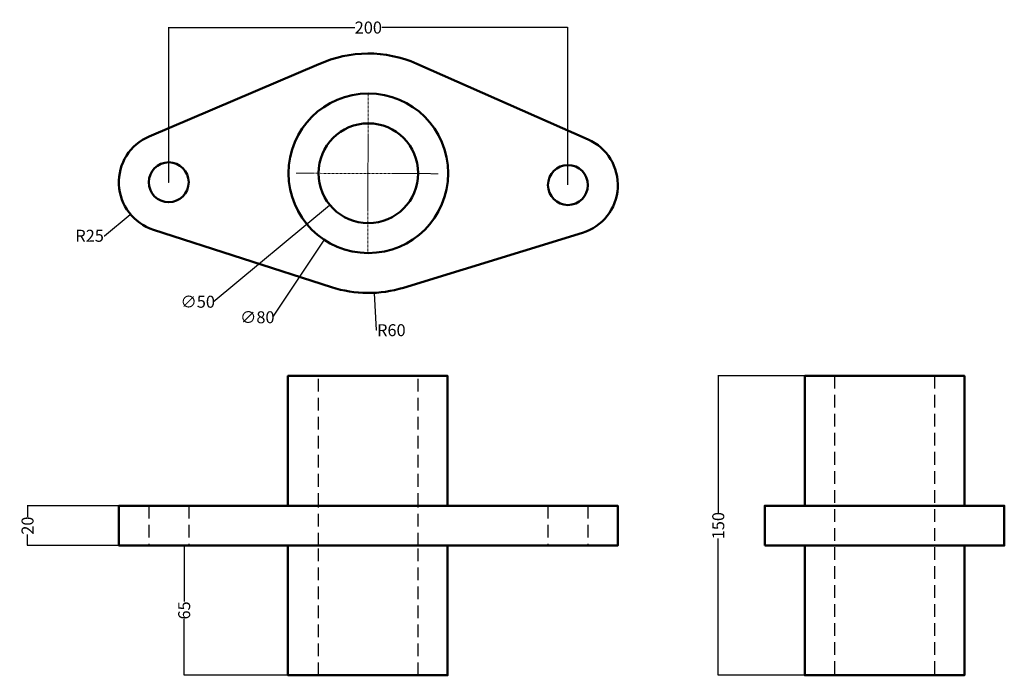
# Model space of a CAD drawing. Units: millimetres. Extents: x 110 to 603, y -63 to 265.
import ezdxf

# ---------------------------------------------------------------- set-up
doc = ezdxf.new("R2010")
doc.units = ezdxf.units.MM
doc.header["$MEASUREMENT"] = 0
doc.linetypes.add('CENTER', pattern=[2, 1.25, -0.25, 0.25, -0.25])
doc.linetypes.add('HIDDEN', pattern=[9.525, 6.35, -3.175])
for name, color, linetype, lineweight in [('M-CNTR', 4, 'CENTER', 18), ('M-DIMS', 2, 'Continuous', 25), ('M-HIDN', 1, 'HIDDEN', 25), ('M-OUTL', 7, 'Continuous', 50)]:
    doc.layers.add(name, color=color, linetype=linetype, lineweight=lineweight)
doc.styles.get("Standard").update_dxf_attribs({"font": 'arial.ttf'})
doc.dimstyles.get("Standard").update_dxf_attribs({"dimtxt": 6, "dimasz": 0.18, "dimexe": 0.18, "dimexo": 0.0625, "dimgap": 0.09, "dimtad": 0, "dimtoh": 1, "dimdec": 0, "dimzin": 0, "dimdsep": 46, "dimtxsty": 'Standard', "dimcen": 0.09, "dimadec": 0, "dimazin": 0, "dimtfac": 1, "dimtdec": 0, "dimtofl": 0, "dimtmove": 0, "dimatfit": 3, "dimfxl": 1, "dimtolj": 1, "dimtzin": 0, "dimarcsym": 0})

# ---------------------------------------------------------------- blocks, each defined once
blk = doc.blocks.new('*D1')
at = {"layer": 'Defpoints', "color": 0, "transparency": 16777216}
for p in [(384.64, 261.41), (184.64, 183.88), (384.64, 182.49)]:
    blk.add_point(p, dxfattribs=at)
at = {"layer": 'M-DIMS', "color": 0, "lineweight": -2, "transparency": 16777216}
for p, q in [((184.64, 183.94), (184.64, 261.59)), ((384.64, 182.55), (384.64, 261.59)), ((184.82, 261.41), (277.88, 261.41)), ((384.46, 261.41), (291.4, 261.41))]:
    blk.add_line(p, q, dxfattribs=at)
at = {"layer": 'M-DIMS', "color": 0, "transparency": 16777216}
for points in [[(184.82, 261.44), (184.82, 261.38), (184.64, 261.41)], [(384.46, 261.44), (384.46, 261.38), (384.64, 261.41)]]:
    blk.add_solid(points, dxfattribs=at)
at = {"layer": 'M-DIMS', "color": 0, "transparency": 16777216, "insert": (284.64, 261.41), "char_height": 6, "attachment_point": 5}
blk.add_mtext('\\A1;200', dxfattribs=at)
blk = doc.blocks.new('*D2')
at = {"layer": 'Defpoints', "color": 0, "transparency": 16777216}
for p in [(184.64, 183.88), (165.43, 167.88)]:
    blk.add_point(p, dxfattribs=at)
at = {"layer": 'M-DIMS', "color": 0, "lineweight": -2, "transparency": 16777216}
for p, q in [((184.55, 183.88), (184.73, 183.88)), ((184.64, 183.79), (184.64, 183.97)), ((152.45, 157.07), (165.29, 167.77)), ((152.27, 157.07), (152.45, 157.07))]:
    blk.add_line(p, q, dxfattribs=at)
at = {"layer": 'M-DIMS', "color": 0, "transparency": 16777216}
blk.add_solid([(165.27, 167.79), (165.31, 167.74), (165.43, 167.88)], dxfattribs=at)
at = {"layer": 'M-DIMS', "color": 0, "transparency": 16777216, "insert": (144.99, 157.07), "char_height": 6, "attachment_point": 5}
blk.add_mtext('\\A1;R25', dxfattribs=at)
blk = doc.blocks.new('*D3')
at = {"layer": 'Defpoints', "color": 0, "transparency": 16777216}
for p in [(284.64, 188.4), (287.76, 128.48)]:
    blk.add_point(p, dxfattribs=at)
at = {"layer": 'M-DIMS', "color": 0, "lineweight": -2, "transparency": 16777216}
for p, q in [((284.55, 188.4), (284.73, 188.4)), ((284.64, 188.31), (284.64, 188.49)), ((288.74, 109.76), (287.77, 128.3)), ((288.92, 109.76), (288.74, 109.76))]:
    blk.add_line(p, q, dxfattribs=at)
at = {"layer": 'M-DIMS', "color": 0, "transparency": 16777216}
blk.add_solid([(287.8, 128.3), (287.74, 128.3), (287.76, 128.48)], dxfattribs=at)
at = {"layer": 'M-DIMS', "color": 0, "transparency": 16777216, "insert": (296.17, 109.76), "char_height": 6, "attachment_point": 5}
blk.add_mtext('\\A1;R60', dxfattribs=at)
blk = doc.blocks.new('*D4')
at = {"layer": 'Defpoints', "color": 0, "transparency": 16777216}
for p in [(303.89, 204.35), (265.39, 172.44)]:
    blk.add_point(p, dxfattribs=at)
at = {"layer": 'M-DIMS', "color": 0, "lineweight": -2, "transparency": 16777216}
for p, q in [((284.55, 188.4), (284.73, 188.4)), ((284.64, 188.31), (284.64, 188.49)), ((206.97, 124.02), (265.25, 172.33)), ((206.79, 124.02), (206.97, 124.02))]:
    blk.add_line(p, q, dxfattribs=at)
at = {"layer": 'M-DIMS', "color": 0, "transparency": 16777216}
blk.add_solid([(265.23, 172.35), (265.27, 172.31), (265.39, 172.44)], dxfattribs=at)
at = {"layer": 'M-DIMS', "color": 0, "transparency": 16777216, "insert": (199.15, 124.02), "char_height": 6, "attachment_point": 5}
blk.add_mtext('\\A1;∅50', dxfattribs=at)
blk = doc.blocks.new('*D5')
at = {"layer": 'Defpoints', "color": 0, "transparency": 16777216}
for p in [(306.73, 221.74), (262.54, 155.06)]:
    blk.add_point(p, dxfattribs=at)
at = {"layer": 'M-DIMS', "color": 0, "lineweight": -2, "transparency": 16777216}
for p, q in [((284.55, 188.4), (284.73, 188.4)), ((284.64, 188.31), (284.64, 188.49)), ((236.82, 116.24), (262.44, 154.91)), ((236.64, 116.24), (236.82, 116.24))]:
    blk.add_line(p, q, dxfattribs=at)
at = {"layer": 'M-DIMS', "color": 0, "transparency": 16777216}
blk.add_solid([(262.42, 154.92), (262.47, 154.89), (262.54, 155.06)], dxfattribs=at)
at = {"layer": 'M-DIMS', "color": 0, "transparency": 16777216, "insert": (229, 116.24), "char_height": 6, "attachment_point": 5}
blk.add_mtext('\\A1;∅80', dxfattribs=at)
blk = doc.blocks.new('*D6')
at = {"layer": 'Defpoints', "color": 0, "transparency": 16777216}
for p in [(113.9, 21.82), (167.53, 21.82), (167.53, 1.82)]:
    blk.add_point(p, dxfattribs=at)
at = {"layer": 'M-DIMS', "color": 0, "lineweight": -2, "transparency": 16777216}
for p, q in [((167.46, 21.82), (113.72, 21.82)), ((113.9, 21.64), (113.9, 16.24)), ((113.9, 2), (113.9, 7.39)), ((167.46, 1.82), (113.72, 1.82))]:
    blk.add_line(p, q, dxfattribs=at)
at = {"layer": 'M-DIMS', "color": 0, "transparency": 16777216}
for points in [[(113.87, 21.64), (113.93, 21.64), (113.9, 21.82)], [(113.87, 2), (113.93, 2), (113.9, 1.82)]]:
    blk.add_solid(points, dxfattribs=at)
at = {"layer": 'M-DIMS', "color": 0, "transparency": 16777216, "insert": (113.9, 11.82), "char_height": 6, "attachment_point": 5, "rotation": 90}
blk.add_mtext('\\A1;20', dxfattribs=at)
blk = doc.blocks.new('*D7')
at = {"layer": 'Defpoints', "color": 0, "transparency": 16777216}
for p in [(244.32, 1.82), (192.38, -63.18), (244.32, -63.18)]:
    blk.add_point(p, dxfattribs=at)
at = {"layer": 'M-DIMS', "color": 0, "lineweight": -2, "transparency": 16777216}
for p, q in [((244.26, 1.82), (192.2, 1.82)), ((192.38, 1.64), (192.38, -26.26)), ((192.38, -63), (192.38, -35.11)), ((244.26, -63.18), (192.2, -63.18))]:
    blk.add_line(p, q, dxfattribs=at)
at = {"layer": 'M-DIMS', "color": 0, "transparency": 16777216}
for points in [[(192.35, 1.64), (192.41, 1.64), (192.38, 1.82)], [(192.35, -63), (192.41, -63), (192.38, -63.18)]]:
    blk.add_solid(points, dxfattribs=at)
at = {"layer": 'M-DIMS', "color": 0, "transparency": 16777216, "insert": (192.38, -30.68), "char_height": 6, "attachment_point": 5, "rotation": 90}
blk.add_mtext('\\A1;65', dxfattribs=at)
blk = doc.blocks.new('*D8')
at = {"layer": 'Defpoints', "color": 0, "transparency": 16777216}
for p in [(543.27, 86.82), (459.96, -63.18), (543.27, -63.18)]:
    blk.add_point(p, dxfattribs=at)
at = {"layer": 'M-DIMS', "color": 0, "lineweight": -2, "transparency": 16777216}
for p, q in [((543.21, 86.82), (459.78, 86.82)), ((459.96, 86.64), (459.96, 18.24)), ((459.96, -63), (459.96, 5.39)), ((543.21, -63.18), (459.78, -63.18))]:
    blk.add_line(p, q, dxfattribs=at)
at = {"layer": 'M-DIMS', "color": 0, "transparency": 16777216}
for points in [[(459.93, 86.64), (459.99, 86.64), (459.96, 86.82)], [(459.93, -63), (459.99, -63), (459.96, -63.18)]]:
    blk.add_solid(points, dxfattribs=at)
at = {"layer": 'M-DIMS', "color": 0, "transparency": 16777216, "insert": (459.96, 11.82), "char_height": 6, "attachment_point": 5, "rotation": 90}
blk.add_mtext('\\A1;150', dxfattribs=at)

msp = doc.modelspace()

# ---------------------------------------------------------------- linework, layer by layer
at = {"layer": 'M-CNTR'}
for p, q in [((284.58, 228.4), (284.33, 148.4)), ((248.5, 188.4), (319.7, 188.18))]:
    msp.add_line(p, q, dxfattribs=at)
at = {"layer": 'M-HIDN'}
for p, q in [((518.27, 86.82), (518.27, -63.18)), ((568.27, 86.82), (568.27, -63.18)), ((174.64, 21.82), (174.64, 1.82)), ((194.64, 21.82), (194.64, 1.82)), ((374.64, 21.82), (374.64, 1.82)), ((394.64, 21.82), (394.64, 1.82))]:
    msp.add_line(p, q, dxfattribs=at)
for points in [[(259.64, -63.18), (259.64, 1.82), (259.64, 21.82), (259.64, 86.82)], [(309.64, -63.18), (309.64, 1.82), (309.64, 21.82), (309.64, 86.82)]]:
    msp.add_lwpolyline(points, dxfattribs=at)
at = {"layer": 'M-OUTL'}
msp.add_lwpolyline([(174.85, 206.89, 0.69424), (176.96, 160.09), (266.22, 131.3, 0.153687), (302.25, 131.04), (391.98, 158.59, 0.69437), (394.74, 205.36), (308.88, 243.28, 0.213721), (259.83, 243.03)], format="xyb", close=True, dxfattribs=at)
for points in [[(244.32, 21.82), (244.32, 86.82), (324.32, 86.82), (324.32, 21.82)], [(503.27, 21.82), (503.27, 86.82), (583.27, 86.82), (583.27, 21.82)], [(244.32, 1.82), (244.32, -63.18), (324.32, -63.18), (324.32, 1.82), (367.19, 1.82)], [(503.27, 1.82), (503.27, -63.18), (583.27, -63.18), (583.27, 1.82)]]:
    msp.add_lwpolyline(points, dxfattribs=at)
for points in [[(159.64, 21.82), (159.64, 1.82), (409.64, 1.82), (409.64, 21.82)], [(483.27, 1.82), (603.27, 1.82), (603.27, 21.82), (483.27, 21.82)]]:
    msp.add_lwpolyline(points, close=True, dxfattribs=at)
for centre, radius in [((284.64, 188.4), 40), ((284.64, 188.4), 25), ((184.64, 183.88), 10), ((384.64, 182.49), 10)]:
    msp.add_circle(centre, radius, dxfattribs=at)

# ---------------------------------------------------------------- dimensions: what is measured, and where the dimension line sits
at = {"layer": 'M-DIMS'}
dim = msp.add_linear_dim(base=(384.64, 261.41), p1=(184.64, 183.88), p2=(384.64, 182.49), dimstyle='Standard', override={"dimclrd": 0, "dimclre": 0, "dimclrt": 0}, dxfattribs=at)
dim.commit()
dim.dimension.update_dxf_attribs({"geometry": '*D1', "text_midpoint": (284.64, 261.41)})
for p1, p2, picture, middle in [((306.73, 221.74), (262.54, 155.06), '*D5', (229, 116.24)), ((303.89, 204.35), (265.39, 172.44), '*D4', (199.15, 124.02))]:
    dim = msp.add_diameter_dim_2p(p1=p1, p2=p2, dimstyle='Standard', override={"dimclrd": 0, "dimclre": 0, "dimclrt": 0}, dxfattribs=at)
    dim.commit()
    dim.dimension.update_dxf_attribs({"geometry": picture, "text_midpoint": middle, "dimtype": 163})
for center, mpoint, picture, middle in [((284.64, 188.4), (287.76, 128.48), '*D3', (296.17, 109.76)), ((184.64, 183.88), (165.43, 167.88), '*D2', (144.99, 157.07))]:
    dim = msp.add_radius_dim(center=center, mpoint=mpoint, dimstyle='Standard', override={"dimclrd": 0, "dimclre": 0, "dimclrt": 0}, dxfattribs=at)
    dim.commit()
    dim.dimension.update_dxf_attribs({"geometry": picture, "text_midpoint": middle, "dimtype": 164})
for base, p1, p2, picture, middle in [((459.96, -63.18), (543.27, 86.82), (543.27, -63.18), '*D8', (459.96, 11.82)), ((113.9, 21.82), (167.53, 1.82), (167.53, 21.82), '*D6', (113.9, 11.82)), ((192.38, -63.18), (244.32, 1.82), (244.32, -63.18), '*D7', (192.38, -30.68))]:
    dim = msp.add_linear_dim(base=base, p1=p1, p2=p2, angle=90, dimstyle='Standard', override={"dimclrd": 0, "dimclre": 0, "dimclrt": 0}, dxfattribs=at)
    dim.commit()
    dim.dimension.update_dxf_attribs({"geometry": picture, "text_midpoint": middle})

doc.saveas('drawing.dxf')
